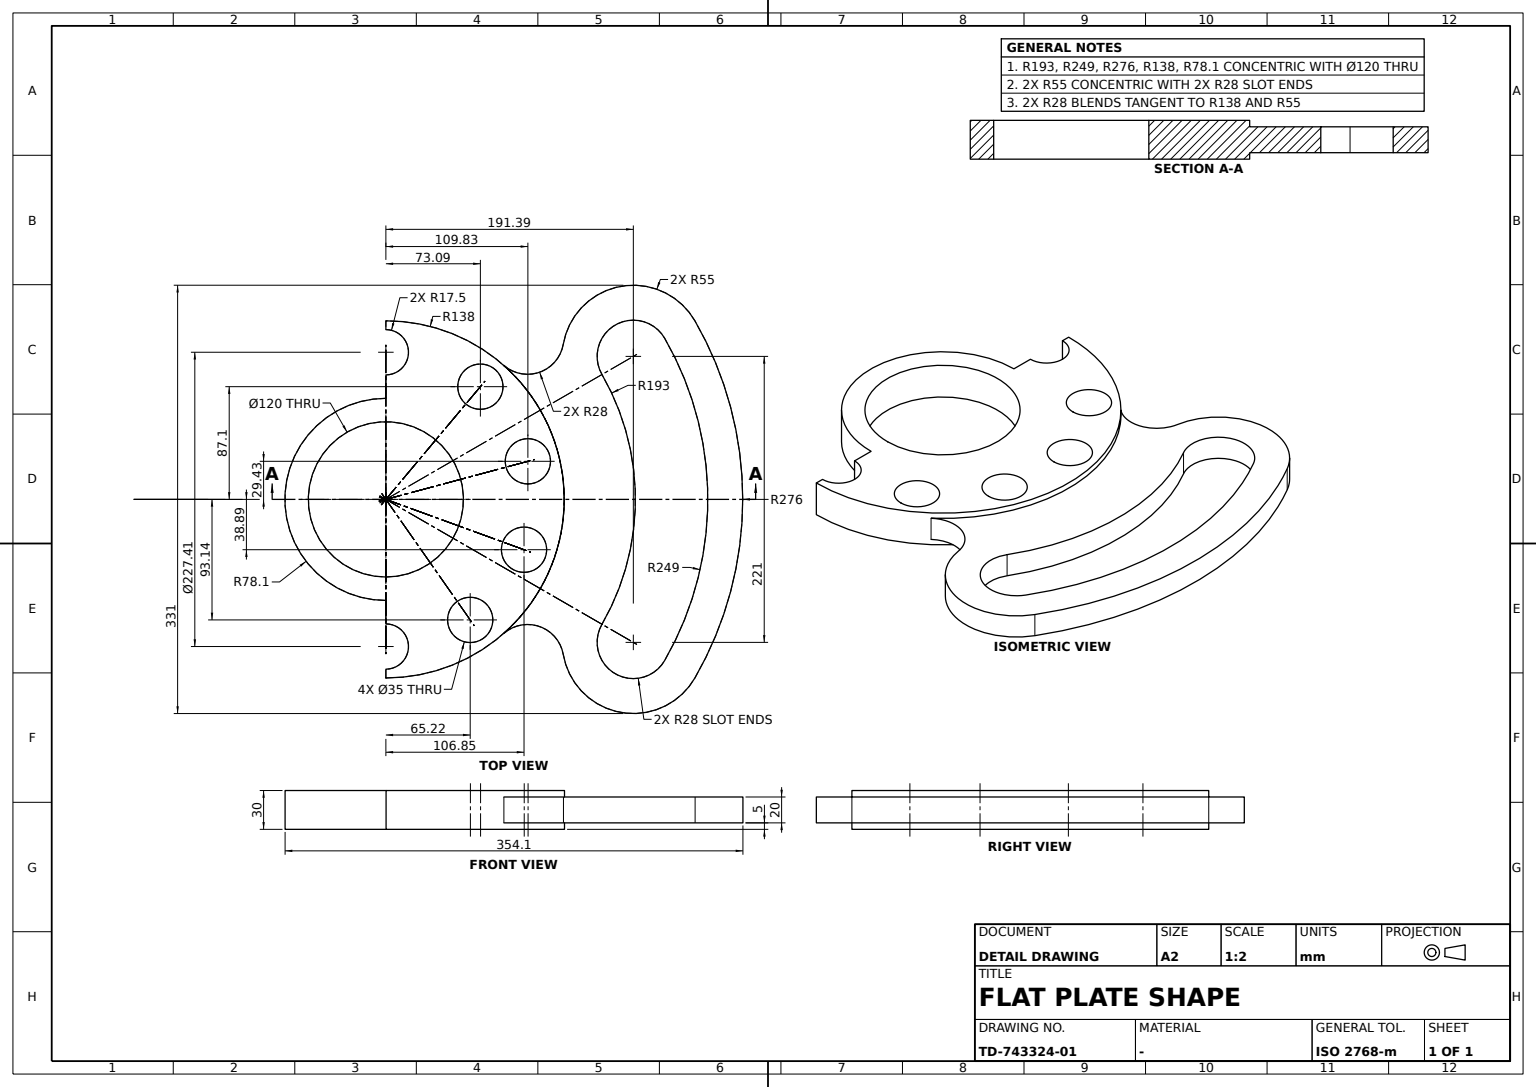
CATIA V5 part; units mm, degrees
sketch "Sketch1" plane through (0, 0, 0) normal (0, 0, 1) x (1, 0, 0)
  arc A0 (138, 0) -> (103.6385, 91.1212) centre (0, 0) ccw
  line L0 (64.0312, 110.9054) -> (-70.4344, -121.9959) construction
  point P0 (64.0312, 110.9054)
  point P1 (-70.4344, -121.9959)
  point P2 (70.4344, -121.9959)
  point P3 (-64.0312, 110.9054)
  line L1 (-64.0312, 110.9054) -> (70.4344, -121.9959) construction
  arc A1 (110.5, 191.3916) -> (-110.5, 191.3916) centre (0, 0) ccw construction
  point P4 (110.5, 191.3916)
  point P5 (-110.5, 191.3916)
  arc A2 (138, 239.023) -> (119.8875, 137.1987) centre (110.5, 191.3916) cw
  arc A3 (-119.8875, 137.1987) -> (-138, 239.023) centre (-110.5, 191.3916) cw
  arc A4 (-138, 239.023) -> (138, 239.023) centre (0, 0) cw
  arc A5 (119.8875, 137.1987) -> (103.6385, 91.1212) centre (124.6666, 109.6095) ccw
  arc A6 (-119.8875, 137.1987) -> (-103.6385, 91.1212) centre (-124.6666, 109.6095) cw
  line L2 (-138, 0) -> (138, 0)
  arc A7 (-103.6385, 91.1212) -> (-138, 0) centre (0, 0) ccw
  dimension "radius A0" = 138
  dimension "angle y axis L0" = 30
  dimension "radius A5" = 28
  dimension "angle y axis L0" = 30
  constraint coincidence L0 origin
  constraint coincidence P4 L0
  constraint coincidence P5 L1
  constraint coincidence A0 A7
  constraint symmetry P1 P2 y-axis
  constraint symmetry P0 P3 y-axis
  constraint symmetry L0 L1 y-axis
  constraint symmetry A5 A6 y-axis
  constraint tangency A3 A4
  constraint tangency A4 A2
  constraint tangency A2 A5
  constraint concentricity A4 origin
  constraint horizontal L2 x-axis
extrude "Pad1" add sketch "Sketch1" along normal mid plane 20
sketch "Sketch2" plane through (0, 0, 0) normal (0, 0, 1) x (1, 0, 0)
  arc A0 (138, 0) -> (-138, 0) centre (0, 0) ccw
  arc A1 (-78.1025, 0) -> (78.1025, 0) centre (0, 0) ccw
  line L0 (-138, 0) -> (-78.1025, 0)
  point P0 (-138, 0)
  point P1 (78.1025, 0)
  line L1 (78.1025, 0) -> (138, 0)
  dimension "radius A0" = 138
  dimension "radius A1" = 78.1025
  constraint coincidence P0 x-axis
  constraint coincidence L0 P1
  constraint coincidence L0 L1
  constraint horizontal L0 x-axis
  constraint horizontal L1 x-axis
extrude "Pad2" add sketch "Sketch2" along normal mid plane 30
sketch "Sketch3" plane through (0, 0, 15) normal (0, 0, 1) x (1, 0, 0)
  arc A0 (124.5, 215.6403) -> (96.5, 167.1429) centre (110.5, 191.3916) cw
  arc A1 (-96.5, 167.1429) -> (-124.5, 215.6403) centre (-110.5, 191.3916) cw
  arc A2 (96.5, 167.1429) -> (-96.5, 167.1429) centre (0, 0) ccw
  arc A3 (-124.5, 215.6403) -> (124.5, 215.6403) centre (0, 0) cw
  circle A4 centre (0, 0) radius 60
  point P0 (30, 51.9615)
  circle A5 centre (113.7051, 0) radius 17.5
  point P1 (113.7051, 0)
  circle A6 centre (-113.7051, 0) radius 17.5
  circle A7 centre (93.1418, 65.2186) radius 17.5
  circle A8 centre (38.8894, 106.8479) radius 17.5
  circle A9 centre (-29.4291, 109.8307) radius 17.5
  circle A10 centre (-87.1032, 73.0882) radius 17.5
  dimension "radius A1" = 28
  dimension "radius A4" = 60
  dimension "radius A5" = 17.5
  constraint tangency A2 A1
  constraint tangency A1 A3
  constraint tangency A3 A0
  constraint tangency A0 A2
  constraint concentricity A2 origin
  constraint concentricity A3 origin
  constraint coincidence A4 P0
  constraint coincidence P1 x-axis
  constraint symmetry A5 A6 y-axis
extrude "Pocket1" cut sketch "Sketch3" against normal through all and the other way blind 20
